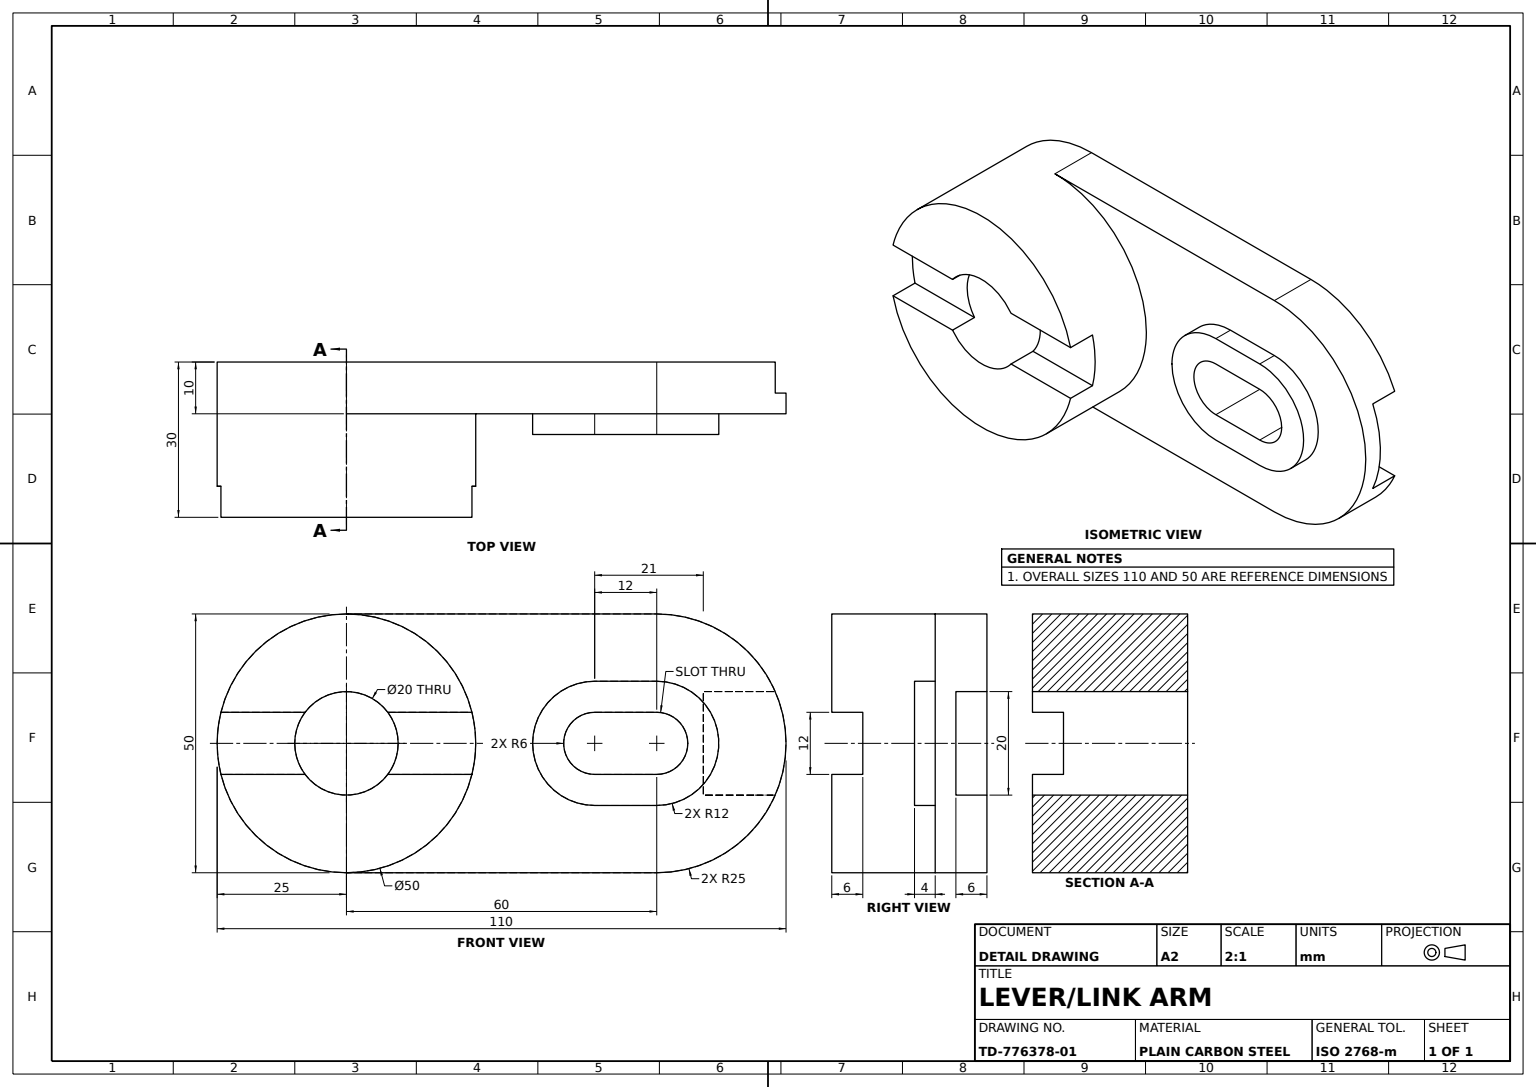
SolidWorks part; units mm, degrees
material "Plain Carbon Steel"
ref_plane "Front Plane" through (0, 0, 0) normal (0, 0, 1) x (1, 0, 0)
ref_plane "Top Plane" through (0, 0, 0) normal (0, 1, 0) x (1, 0, 0)
ref_plane "Right Plane" through (0, 0, 0) normal (1, 0, 0) x (0, 0, -1)
sketch "Arm Profile Sketch" plane through (0, 0, 0) normal (0, 0, 1) x (1, 0, 0)
  line L2 (60, 25) -> (0, 25)
  line L3 (0, 25) -> (0, -25)
  line L4 (0, -25) -> (60, -25)
  arc A0 (60, -25) -> (60, 25) centre (60, 0) ccw
  dimension "D1" = 50
  dimension "D2" = 25
  dimension "D3" = 60
extrude "Arm Plate" add sketch "Arm Profile Sketch" along normal blind 10
sketch "Hub Front Sketch" plane through (0, 0, 10) normal (0, 0, 1) x (1, 0, 0)
  circle A0 centre (0, 0) radius 25
  dimension "D1" = 50
  dimension "D2" = 50
extrude "Hub Boss Front" add sketch "Hub Front Sketch" against normal blind 10
sketch "Hub Back Sketch" plane through (0, 0, 10) normal (0, 0, 1) x (1, 0, 0)
  circle A0 centre (0, 0) radius 25
  dimension "D1" = 50
  dimension "D2" = 50
extrude "Hub Boss Back" add sketch "Hub Back Sketch" along normal blind 20
sketch "Hub Cross Slot Sketch" plane through (0, 0, 30) normal (0, 0, 1) x (1, 0, 0)
  line L0 (25, 0) -> (25, 6)
  line L1 (25, 6) -> (25, -6)
  line L2 (25, -6) -> (8, -6)
  line L3 (-25, -6) -> (-25, 6)
  line L4 (-25, 6) -> (-8, 6)
  line L5 (8, 6) -> (25, 6)
  line L6 (-8, -6) -> (-25, -6)
  arc A0 (-8, -6) -> (8, -6) centre (0, 0) ccw
  arc A1 (0, -25) -> (0, 25) centre (0, 0) ccw construction
  arc A2 (8, 6) -> (-8, 6) centre (0, 0) ccw
  circle A3 centre (0, 0) radius 25 construction
  circle M1 centre (0, 0) radius 25
  dimension "D1" = 20
  dimension "D2" = 10
  dimension "D3" = 8
extrude "Hub Cross Slot" cut sketch "Hub Cross Slot Sketch" against normal blind 6 contours L5 A2 L4 L6 A0 L2 M1
sketch "Bore Sketch" plane through (0, 0, 24) normal (0, 0, 1) x (1, 0, 0)
  circle A0 centre (0, 0) radius 10
  dimension "D1" = 20
  dimension "D2" = 20
extrude "Bore Ø20" cut sketch "Bore Sketch" against normal blind 30
sketch "Slot Boss Sketch" plane through (0, 0, 10) normal (0, 0, 1) x (1, 0, 0)
  line L1 (48, 12) -> (60, 12)
  line L2 (48, -12) -> (60, -12)
  arc A0 (60, -12) -> (60, 12) centre (60, 0) ccw
  arc A1 (48, 12) -> (48, -12) centre (48, 0) ccw
  dimension "D1" = 24
  dimension "D2" = 24
  dimension "D3" = 12
extrude "Slot Boss" add sketch "Slot Boss Sketch" along normal blind 4
sketch "Arm Slot Sketch" plane through (0, 0, 14) normal (0, 0, 1) x (1, 0, 0)
  line L0 (48, 6) -> (60, 6)
  line L2 (60, -6) -> (48, -6)
  arc A0 (60, -6) -> (60, 6) centre (60, 0) ccw
  arc A1 (48, 6) -> (48, -6) centre (48, 0) ccw
  dimension "D1" = 12
  dimension "D2" = 12
  dimension "D3" = 6
extrude "Arm Slot 12mm" cut sketch "Arm Slot Sketch" against normal blind 20
sketch "End Notch Sketch" plane through (0, 0, 0) normal (0, 0, -1) x (-1, 0, 0)
  line L2 (-79, 10) -> (-82.9129, 10)
  line L4 (-82.9129, -10) -> (-79, -10)
  line L5 (-79, 10) -> (-69, 10)
  line L6 (-69, 10) -> (-69, -10)
  line L7 (-69, -10) -> (-79, -10)
  arc A0 (-60, 25) -> (-60, -25) centre (-60, 0) ccw construction
  dimension "D1" = 21
  dimension "D2" = 31
  dimension "D3" = 34.9129
extrude "End Notch" cut sketch "End Notch Sketch" against normal blind 6 and the other way through all
